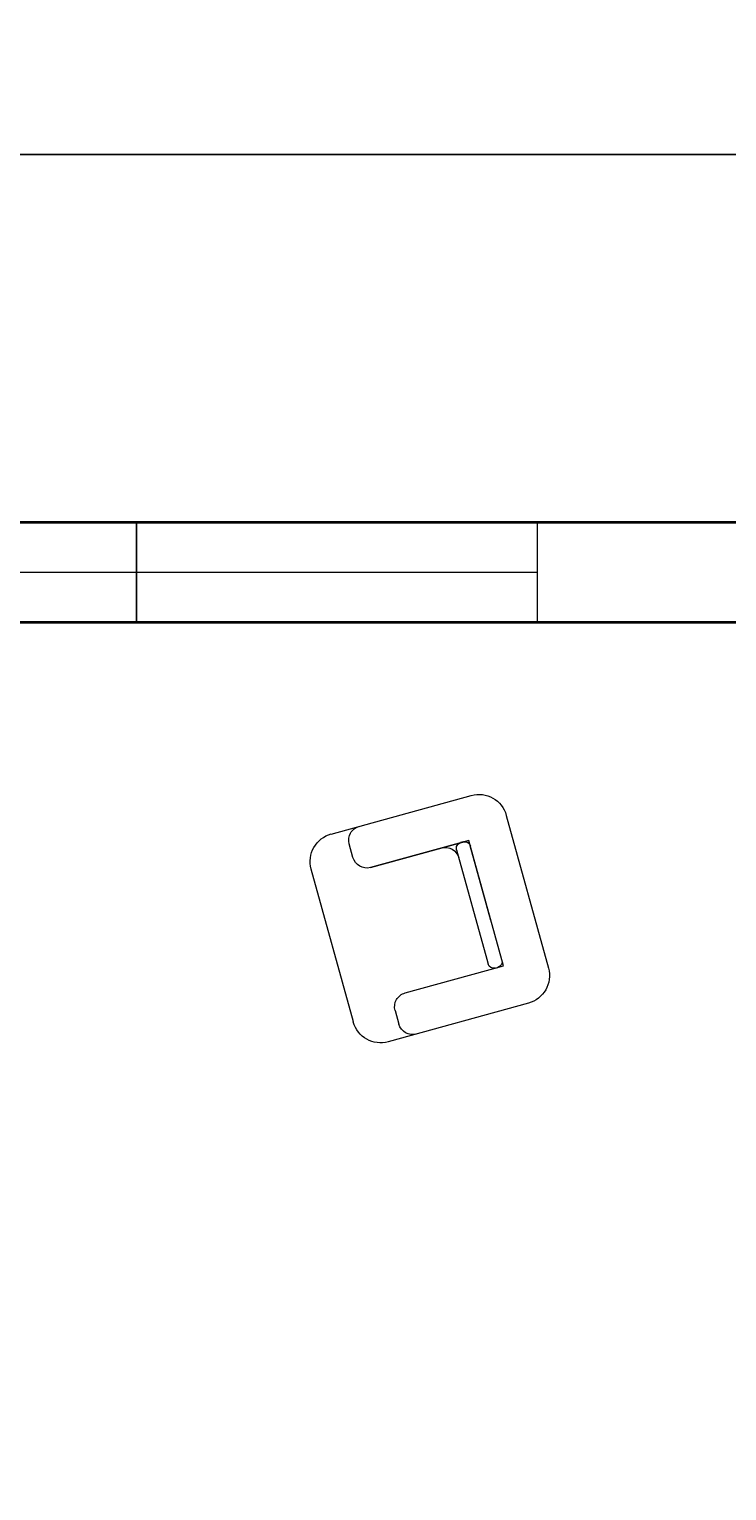
# Model space of a CAD drawing. Units: millimetres. Extents: x 27017497 to 27018854, y 7058029 to 7059154.
# Tile 88 of 91: x 27018399 to 27018462, y 7058503 to 7058634. Entities that reach past the tile are written whole.
import ezdxf

# ---------------------------------------------------------------- set-up
doc = ezdxf.new("R2010")
doc.units = ezdxf.units.MM
for name, color, linetype, lineweight in [('A-ANNO-DIMS', 2, 'Continuous', 18), ('A-FURN', 8, 'Continuous', 18), ('A-GLAZ', 4, 'Continuous', 18), ('A-WALL', 7, 'Continuous', 35)]:
    doc.layers.add(name, color=color, linetype=linetype, lineweight=lineweight)
doc.styles.get("Standard").update_dxf_attribs({"font": 'arial.ttf'})
doc.dimstyles.get("Standard").update_dxf_attribs({"dimtxt": 0.18, "dimasz": 0.18, "dimexe": 0.18, "dimexo": 0.0625, "dimgap": 0.09, "dimtad": 0, "dimtih": 1, "dimtoh": 1, "dimdec": 4, "dimzin": 0, "dimdsep": 46, "dimtxsty": 'Standard', "dimcen": 0.09, "dimadec": 0, "dimazin": 0, "dimtfac": 1, "dimtdec": 4, "dimtofl": 0, "dimtmove": 0, "dimatfit": 3, "dimfxl": 1, "dimtolj": 1, "dimtzin": 0, "dimarcsym": 0})

# ---------------------------------------------------------------- blocks, each defined once
blk = doc.blocks.new('CHAIR-OCCASIONAL')
for p, q in [((19.6, 18.74), (7.02, 22.21)), ((3.87, 20.42), (0.09, 6.71)), ((4.13, 6.92), (7.23, 18.17)), ((5.25, 10.97), (7.23, 18.17)), ((5.25, 10.97), (7.1, 17.68)), ((8.33, 17.34), (5.63, 7.52)), ((16.06, 15.73), (7.23, 18.17)), ((7.23, 18.17), (16.06, 15.73)), ((7.23, 18.17), (16.06, 15.73)), ((7.73, 18.03), (7.97, 17.97)), ((7.73, 18.03), (7.97, 17.97)), ((17.64, 16.63), (17.98, 17.86)), ((17.64, 16.63), (17.98, 17.86)), ((17.6, 1.88), (21.39, 15.6)), ((12.96, 4.48), (4.13, 6.92)), ((4.87, 6.71), (4.63, 6.78)), ((5.63, 7.52), (5.5, 7.07)), ((1.88, 3.56), (14.46, 0.09)), ((13.86, 2.91), (13.52, 1.68))]:
    blk.add_line(p, q)
for centre, radius, start, end in [((6.34, 19.74), 2.56, 74.5879, 164.5879), ((16.74, 18.2), 1.28, 344.5879, 74.5879), ((16.74, 18.2), 1.28, 344.5879, 74.5879), ((18.92, 16.28), 2.56, 344.5879, 74.5879), ((7.59, 17.54), 0.512, 74.5879, 164.5879), ((7.84, 17.47), 0.512, 344.5879, 74.5879), ((9.36, 16.26), 1.28, 74.5879, 164.5879), ((16.4, 16.97), 1.28, 254.5879, 344.5879), ((16.4, 16.97), 1.28, 254.5879, 344.5879), ((2.56, 6.03), 2.56, 164.5879, 254.5879), ((4.76, 7.28), 0.512, 164.5879, 254.5879), ((5.01, 7.21), 0.512, 254.5879, 344.5879), ((12.62, 3.25), 1.28, 344.5879, 74.5879), ((12.28, 2.02), 1.28, 254.5879, 344.5879), ((15.14, 2.56), 2.56, 254.5879, 344.5879)]:
    blk.add_arc(centre, radius, start, end)
blk = doc.blocks.new('WINDOW-SINGLE-LIGHT')
blk.add_lwpolyline([(36, 4.5), (36, 0), (0, 0), (0, 9), (36, 9), (36, 4.5), (0, 4.5)])
blk = doc.blocks.new('*D48')
at = {"layer": 'A-ANNO-DIMS', "color": 0, "lineweight": -2, "transparency": 16777216}
for p, q in [((27018463.5, 7058622.91), (27017497.54, 7058622.91)), ((27017497.72, 7058622.73), (27017497.72, 7058357.75)), ((27017497.72, 7058092.41), (27017497.72, 7058357.39)), ((27018555.13, 7058092.23), (27017497.54, 7058092.23))]:
    blk.add_line(p, q, dxfattribs=at)
at = {"layer": 'A-ANNO-DIMS', "color": 0, "transparency": 16777216}
for points in [[(27017497.69, 7058622.73), (27017497.75, 7058622.73), (27017497.72, 7058622.91)], [(27017497.69, 7058092.41), (27017497.75, 7058092.41), (27017497.72, 7058092.23)]]:
    blk.add_solid(points, dxfattribs=at)
at = {"layer": 'Defpoints', "color": 0, "transparency": 16777216}
for p in [(27018463.56, 7058622.91), (27017497.72, 7058092.23), (27018555.19, 7058092.23)]:
    blk.add_point(p, dxfattribs=at)
at = {"layer": 'A-ANNO-DIMS', "color": 0, "transparency": 16777216, "insert": (27017497.72, 7058357.57), "char_height": 0.18, "attachment_point": 5}
blk.add_mtext('\\A1;530.7', dxfattribs=at)
blk = doc.blocks.new('*D50')
at = {"layer": 'A-ANNO-DIMS', "color": 0, "lineweight": -2, "transparency": 16777216}
for p, q in [((27018223.67, 7058580.91), (27018854.24, 7058580.91)), ((27018854.06, 7058580.73), (27018854.06, 7058511.34)), ((27018854.06, 7058441.59), (27018854.06, 7058510.98)), ((27018223.67, 7058441.41), (27018854.24, 7058441.41))]:
    blk.add_line(p, q, dxfattribs=at)
at = {"layer": 'A-ANNO-DIMS', "color": 0, "transparency": 16777216}
for points in [[(27018854.03, 7058580.73), (27018854.09, 7058580.73), (27018854.06, 7058580.91)], [(27018854.03, 7058441.59), (27018854.09, 7058441.59), (27018854.06, 7058441.41)]]:
    blk.add_solid(points, dxfattribs=at)
at = {"layer": 'Defpoints', "color": 0, "transparency": 16777216}
for p in [(27018223.61, 7058580.91), (27018223.61, 7058441.41), (27018854.06, 7058441.41)]:
    blk.add_point(p, dxfattribs=at)
at = {"layer": 'A-ANNO-DIMS', "color": 0, "transparency": 16777216, "insert": (27018854.06, 7058511.16), "char_height": 0.18, "attachment_point": 5}
blk.add_mtext('\\A1;139.5', dxfattribs=at)
blk = doc.blocks.new('*D52')
at = {"layer": 'A-ANNO-DIMS', "color": 0, "lineweight": -2, "transparency": 16777216}
for p, q in [((27018310.61, 7058589.97), (27018310.61, 7058686.54)), ((27018738.11, 7058589.97), (27018738.11, 7058686.54)), ((27018310.79, 7058686.36), (27018523.96, 7058686.36)), ((27018737.93, 7058686.36), (27018524.75, 7058686.36))]:
    blk.add_line(p, q, dxfattribs=at)
at = {"layer": 'A-ANNO-DIMS', "color": 0, "transparency": 16777216}
for points in [[(27018310.79, 7058686.39), (27018310.79, 7058686.33), (27018310.61, 7058686.36)], [(27018737.93, 7058686.39), (27018737.93, 7058686.33), (27018738.11, 7058686.36)]]:
    blk.add_solid(points, dxfattribs=at)
at = {"layer": 'Defpoints', "color": 0, "transparency": 16777216}
for p in [(27018738.11, 7058686.36), (27018310.61, 7058589.91), (27018738.11, 7058589.91)]:
    blk.add_point(p, dxfattribs=at)
at = {"layer": 'A-ANNO-DIMS', "color": 0, "transparency": 16777216, "insert": (27018524.36, 7058686.36), "char_height": 0.18, "attachment_point": 5}
blk.add_mtext('\\A1;427.5', dxfattribs=at)

msp = doc.modelspace()

# ---------------------------------------------------------------- linework, layer by layer
at = {"layer": 'A-WALL'}
for p, q in [((27018738.106, 7058589.912), (27018310.606, 7058589.912)), ((27018729.106, 7058580.912), (27018319.606, 7058580.912))]:
    msp.add_line(p, q, dxfattribs=at)

# ---------------------------------------------------------------- block references
at = {"layer": 'A-FURN', "extrusion": (0, 0, -1), "zscale": -1}
msp.add_blockref('CHAIR-OCCASIONAL', (-27018446.197, 7058543.199), dxfattribs=at)
at = {"layer": 'A-GLAZ', "extrusion": (0, 0, -1), "zscale": -1}
for p in [(-27018409.137, 7058580.929), (-27018445.136, 7058580.927)]:
    msp.add_blockref('WINDOW-SINGLE-LIGHT', p, dxfattribs=at)

# ---------------------------------------------------------------- dimensions: what is measured, and where the dimension line sits
at = {"layer": 'A-ANNO-DIMS'}
dim = msp.add_linear_dim(base=(27018738.106, 7058686.362), p1=(27018310.606, 7058589.912), p2=(27018738.106, 7058589.912), dimstyle='Standard', override={"dimdec": 1, "dimlfac": 1, "dimrnd": 0, "dimzin": 0, "dimdsep": 46, "dimlunit": 2}, dxfattribs=at)
dim.commit()
dim.dimension.update_dxf_attribs({"geometry": '*D52', "text_midpoint": (27018524.356, 7058686.362)})
for base, p1, p2, picture, middle in [((27017497.716, 7058092.23), (27018463.561, 7058622.912), (27018555.192, 7058092.23), '*D48', (27017497.716, 7058357.571)), ((27018854.056, 7058441.412), (27018223.606, 7058580.912), (27018223.606, 7058441.412), '*D50', (27018854.056, 7058511.162))]:
    dim = msp.add_linear_dim(base=base, p1=p1, p2=p2, angle=90, dimstyle='Standard', override={"dimdec": 1, "dimlfac": 1, "dimrnd": 0, "dimzin": 0, "dimdsep": 46, "dimlunit": 2}, dxfattribs=at)
    dim.commit()
    dim.dimension.update_dxf_attribs({"geometry": picture, "text_midpoint": middle})

doc.saveas('drawing.dxf')
